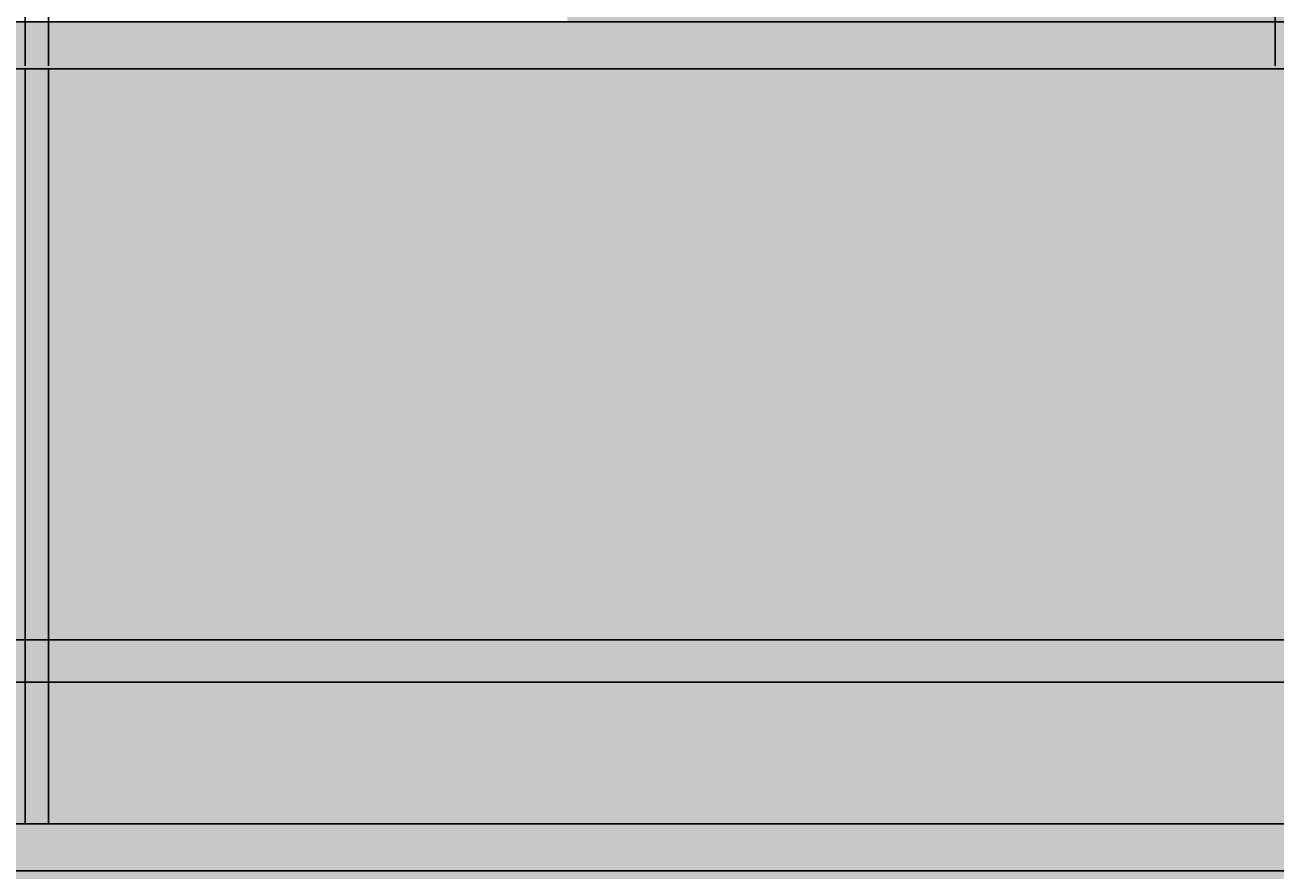
# Model space of a CAD drawing. Units: inches. Extents: x 4508 to 4723, y 847 to 1020.
# Tile 5 of 32: x 4577 to 4604, y 887 to 905. Entities that reach past the tile are written whole.
import ezdxf

# ---------------------------------------------------------------- set-up
doc = ezdxf.new("R2010")
doc.units = ezdxf.units.IN
for name, color, linetype, lineweight in [('A-ANNO-DIMS', 2, 'Continuous', 18), ('A-ANNO-NPLT', 8, 'Continuous', 13), ('A-FURN', 8, 'Continuous', 25), ('A-WALL-PATT', 254, 'Continuous', 13)]:
    doc.layers.add(name, color=color, linetype=linetype, lineweight=lineweight)
doc.styles.get("Standard").update_dxf_attribs({"font": 'arial.ttf'})
doc.dimstyles.get("Standard").update_dxf_attribs({"dimtxt": 0.18, "dimasz": 0.18, "dimexe": 0.18, "dimexo": 0.0625, "dimgap": 0.09, "dimtad": 0, "dimtih": 1, "dimtoh": 1, "dimdec": 4, "dimzin": 0, "dimdsep": 46, "dimtxsty": 'Standard', "dimcen": 0.09, "dimadec": 0, "dimazin": 0, "dimtfac": 1, "dimtdec": 4, "dimtofl": 0, "dimtmove": 0, "dimatfit": 3, "dimfxl": 1, "dimtolj": 1, "dimtzin": 0, "dimarcsym": 0})

# ---------------------------------------------------------------- blocks, each defined once
blk = doc.blocks.new('*D28')
at = {"layer": 'A-ANNO-DIMS', "color": 0, "lineweight": -2, "transparency": 16777216}
for p, q in [((4577.494, 903.809), (4577.494, 1002.877)), ((4577.994, 903.809), (4577.994, 1002.877)), ((4577.314, 1002.697), (4577.134, 1002.697)), ((4578.174, 1002.697), (4578.354, 1002.697))]:
    blk.add_line(p, q, dxfattribs=at)
at = {"layer": 'A-ANNO-DIMS', "color": 0, "lineweight": 9, "transparency": 16777216}
for points in [[(4577.314, 1002.727), (4577.314, 1002.667), (4577.494, 1002.697)], [(4578.174, 1002.727), (4578.174, 1002.667), (4577.994, 1002.697)]]:
    blk.add_solid(points, dxfattribs=at)
at = {"layer": 'Defpoints', "color": 0, "lineweight": 9, "transparency": 16777216}
for p in [(4577.994, 1002.697), (4577.494, 903.747), (4577.994, 903.747)]:
    blk.add_point(p, dxfattribs=at)
at = {"layer": 'A-ANNO-DIMS', "color": 0, "transparency": 16777216, "insert": (4578.608, 1002.697), "char_height": 0.18, "attachment_point": 5}
blk.add_mtext('\\A1;0.5', dxfattribs=at)
blk = doc.blocks.new('*D29')
at = {"layer": 'A-ANNO-DIMS', "color": 0, "lineweight": -2, "transparency": 16777216}
for p, q in [((4577.994, 903.809), (4577.994, 1002.877)), ((4603.994, 903.809), (4603.994, 1002.877)), ((4578.174, 1002.697), (4590.773, 1002.697)), ((4603.814, 1002.697), (4591.214, 1002.697))]:
    blk.add_line(p, q, dxfattribs=at)
at = {"layer": 'A-ANNO-DIMS', "color": 0, "lineweight": 9, "transparency": 16777216}
for points in [[(4578.174, 1002.727), (4578.174, 1002.667), (4577.994, 1002.697)], [(4603.814, 1002.727), (4603.814, 1002.667), (4603.994, 1002.697)]]:
    blk.add_solid(points, dxfattribs=at)
at = {"layer": 'Defpoints', "color": 0, "lineweight": 9, "transparency": 16777216}
for p in [(4603.994, 1002.697), (4577.994, 903.747), (4603.994, 903.747)]:
    blk.add_point(p, dxfattribs=at)
at = {"layer": 'A-ANNO-DIMS', "color": 0, "transparency": 16777216, "insert": (4590.994, 1002.697), "char_height": 0.18, "attachment_point": 5}
blk.add_mtext('\\A1;26', dxfattribs=at)
blk = doc.blocks.new('*D32')
at = {"layer": 'A-ANNO-DIMS', "color": 0, "lineweight": -2, "transparency": 16777216}
for p, q in [((4604.431, 890.747), (4532.864, 890.747)), ((4533.044, 890.567), (4533.044, 889.429)), ((4533.044, 887.927), (4533.044, 889.065)), ((4604.431, 887.747), (4532.864, 887.747))]:
    blk.add_line(p, q, dxfattribs=at)
at = {"layer": 'A-ANNO-DIMS', "color": 0, "lineweight": 9, "transparency": 16777216}
for points in [[(4533.014, 890.567), (4533.074, 890.567), (4533.044, 890.747)], [(4533.014, 887.927), (4533.074, 887.927), (4533.044, 887.747)]]:
    blk.add_solid(points, dxfattribs=at)
at = {"layer": 'Defpoints', "color": 0, "lineweight": 9, "transparency": 16777216}
for p in [(4533.044, 890.747), (4604.494, 890.747), (4604.494, 887.747)]:
    blk.add_point(p, dxfattribs=at)
at = {"layer": 'A-ANNO-DIMS', "color": 0, "transparency": 16777216, "insert": (4533.044, 889.247), "char_height": 0.18, "attachment_point": 5}
blk.add_mtext('\\A1;3', dxfattribs=at)
blk = doc.blocks.new('*D41')
at = {"layer": 'A-ANNO-DIMS', "color": 0, "lineweight": -2, "transparency": 16777216}
for p, q in [((4533.044, 891.643), (4533.044, 891.823)), ((4533.044, 891.823), (4533.224, 891.823)), ((4616.47, 891.643), (4532.864, 891.643)), ((4533.044, 890.927), (4533.044, 891.463)), ((4608.499, 890.747), (4532.864, 890.747))]:
    blk.add_line(p, q, dxfattribs=at)
at = {"layer": 'A-ANNO-DIMS', "color": 0, "lineweight": 9, "transparency": 16777216}
for points in [[(4533.014, 891.463), (4533.074, 891.463), (4533.044, 891.643)], [(4533.014, 890.927), (4533.074, 890.927), (4533.044, 890.747)]]:
    blk.add_solid(points, dxfattribs=at)
at = {"layer": 'Defpoints', "color": 0, "lineweight": 9, "transparency": 16777216}
for p in [(4533.044, 891.643), (4616.533, 891.643), (4608.562, 890.747)]:
    blk.add_point(p, dxfattribs=at)
at = {"layer": 'A-ANNO-DIMS', "color": 0, "transparency": 16777216, "insert": (4533.547, 891.823), "char_height": 0.18, "attachment_point": 5}
blk.add_mtext('\\A1;0.90', dxfattribs=at)

msp = doc.modelspace()

# ---------------------------------------------------------------- hatches: boundary and pattern name
at = {"layer": 'A-WALL-PATT', "transparency": 33554508}
h = msp.add_hatch(color=256, dxfattribs=at)
h.dxf.hatch_style = 1
h.paths.add_polyline_path([(4661.6706, 954.043, -0.3739004), (4658.5765, 957.6021, -1), (4665.7646, 957.6021, -0.3739004), (4662.6706, 954.043), (4662.6706, 944.4021, -0.2114781), (4670.3062, 945.0869), (4670.3062, 968.0592, -0.4632086), (4663.3246, 973.9783, -0.4632086), (4670.3062, 979.8975), (4670.3062, 994.7469), (4588.9938, 994.7469), (4588.9938, 904.7469), (4657.9938, 904.7469), (4657.9938, 886.7469), (4549.9938, 886.7469), (4549.9938, 878.7469), (4693.9938, 878.7469), (4693.9938, 994.7469), (4671.8062, 994.7469), (4671.8062, 979.4411, -0.2941682), (4675.3246, 973.9783, -0.2941682), (4671.8062, 968.5156), (4671.8062, 944.4278, -0.2741114), (4676.7298, 936.1217, -0.2741114), (4671.8062, 927.8155), (4671.8062, 907.6998, -0.3779645), (4677.0562, 901.7469, -0.3779645), (4671.8062, 895.7939), (4671.8062, 883.7469), (4670.3062, 883.7469), (4670.3062, 895.7939, -0.3779645), (4665.0562, 901.7469, -0.3779645), (4670.3062, 907.6998), (4670.3062, 927.1564, -0.2114781), (4662.6706, 927.8412), (4662.6706, 918.2003, -0.3739004), (4665.7646, 914.6412, -1), (4658.5765, 914.6412, -0.3739004), (4661.6706, 918.2003), (4661.6706, 928.4807, -0.2391825), (4657.7936, 936.1217, -0.2391825), (4661.6706, 943.7626)])
at = {"layer": 'A-WALL-PATT', "transparency": 33554681}
h = msp.add_hatch(color=256, dxfattribs=at)
h.dxf.hatch_style = 1
h.paths.add_polyline_path([(4577.4938, 903.7469), (4550.9938, 903.7469), (4550.9938, 887.7469), (4577.4938, 887.7469)], flags=0)
h.paths.add_polyline_path([(4603.9938, 903.7469), (4577.9938, 903.7469), (4577.9938, 887.7469), (4603.9938, 887.7469)], flags=0)
h.paths.add_polyline_path([(4656.9938, 903.7469), (4630.9938, 903.7469), (4630.9938, 887.7469), (4656.9938, 887.7469)], flags=0)
h.paths.add_polyline_path([(4657.9938, 904.7469), (4549.9938, 904.7469), (4549.9938, 886.7469), (4657.9938, 886.7469)])
h.paths.add_polyline_path([(4656.9938, 903.7469), (4656.9938, 887.7469), (4550.9938, 887.7469), (4550.9938, 903.7469)], flags=16)
h = msp.add_hatch(color=256, dxfattribs=at)
h.dxf.hatch_style = 1
h.paths.add_polyline_path([(4577.4938, 903.7469), (4550.9938, 903.7469), (4550.9938, 887.7469), (4577.4938, 887.7469)])
h.paths.add_polyline_path([(4603.9938, 903.7469), (4577.9938, 903.7469), (4577.9938, 887.7469), (4603.9938, 887.7469)])
h.paths.add_polyline_path([(4656.9938, 903.7469), (4630.9938, 903.7469), (4630.9938, 887.7469), (4656.9938, 887.7469)])
h = msp.add_hatch(color=256, dxfattribs=at)
h.dxf.hatch_style = 1
h.paths.add_polyline_path([(4604.4938, 903.7469), (4603.9938, 903.7469), (4603.9938, 887.7469), (4604.4938, 887.7469)])
h.paths.add_polyline_path([(4630.9938, 903.7469), (4630.4938, 903.7469), (4630.4938, 887.7469), (4630.9938, 887.7469)])
h.paths.add_polyline_path([(4577.9938, 903.7469), (4577.4938, 903.7469), (4577.4938, 887.7469), (4577.9938, 887.7469)])

# ---------------------------------------------------------------- linework, layer by layer
at = {"layer": 'A-ANNO-NPLT'}
msp.add_point((4577.4938, 895.7469), dxfattribs=at)
at = {"layer": 'A-FURN'}
for p, q in [((4577.4938, 903.7469), (4577.4938, 887.7469)), ((4577.9938, 903.7469), (4577.9938, 887.7469))]:
    msp.add_line(p, q, dxfattribs=at)
for points in [[(4657.9938, 886.7469), (4549.9938, 886.7469), (4549.9938, 904.7469), (4657.9938, 904.7469)], [(4656.9938, 887.7469), (4550.9938, 887.7469), (4550.9938, 903.7469), (4656.9938, 903.7469)]]:
    msp.add_lwpolyline(points, close=True, dxfattribs=at)

# ---------------------------------------------------------------- dimensions: what is measured, and where the dimension line sits
at = {"layer": 'A-ANNO-DIMS'}
for base, p1, p2, override, picture, middle in [((4577.9938, 1002.6969), (4577.4938, 903.7469), (4577.9938, 903.7469), {"dimdec": 1, "dimlfac": 1, "dimrnd": 0, "dimzin": 0, "dimdsep": 46, "dimlunit": 2}, '*D28', (4578.6083, 1002.6969)), ((4603.9938, 1002.6969), (4577.9938, 903.7469), (4603.9938, 903.7469), {"dimdec": 0, "dimlfac": 1, "dimrnd": 0, "dimzin": 0, "dimdsep": 46, "dimlunit": 2}, '*D29', (4590.9938, 1002.6969))]:
    dim = msp.add_linear_dim(base=base, p1=p1, p2=p2, dimstyle='Standard', override=override, dxfattribs=at)
    dim.commit()
    dim.dimension.update_dxf_attribs({"geometry": picture, "text_midpoint": middle})
for base, p1, p2, override, picture, middle in [((4533.0438, 891.6433), (4608.5617, 890.7469), (4616.5328, 891.6433), {"dimdec": 2, "dimlfac": 1, "dimrnd": 0, "dimzin": 0, "dimdsep": 46, "dimlunit": 2}, '*D41', (4533.5473, 891.8233)), ((4533.0438, 890.7469), (4604.4938, 887.7469), (4604.4938, 890.7469), {"dimdec": 0, "dimlfac": 1, "dimrnd": 0, "dimzin": 0, "dimdsep": 46, "dimlunit": 2}, '*D32', (4533.0438, 889.2469))]:
    dim = msp.add_linear_dim(base=base, p1=p1, p2=p2, angle=90, dimstyle='Standard', override=override, dxfattribs=at)
    dim.commit()
    dim.dimension.update_dxf_attribs({"geometry": picture, "text_midpoint": middle})

doc.saveas('drawing.dxf')
